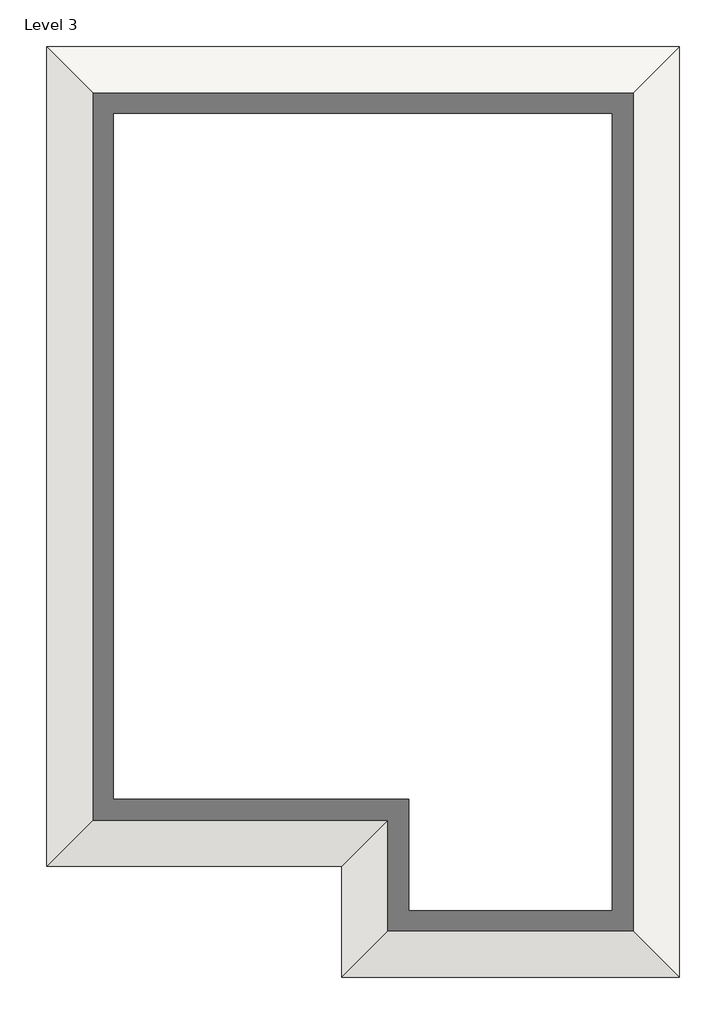
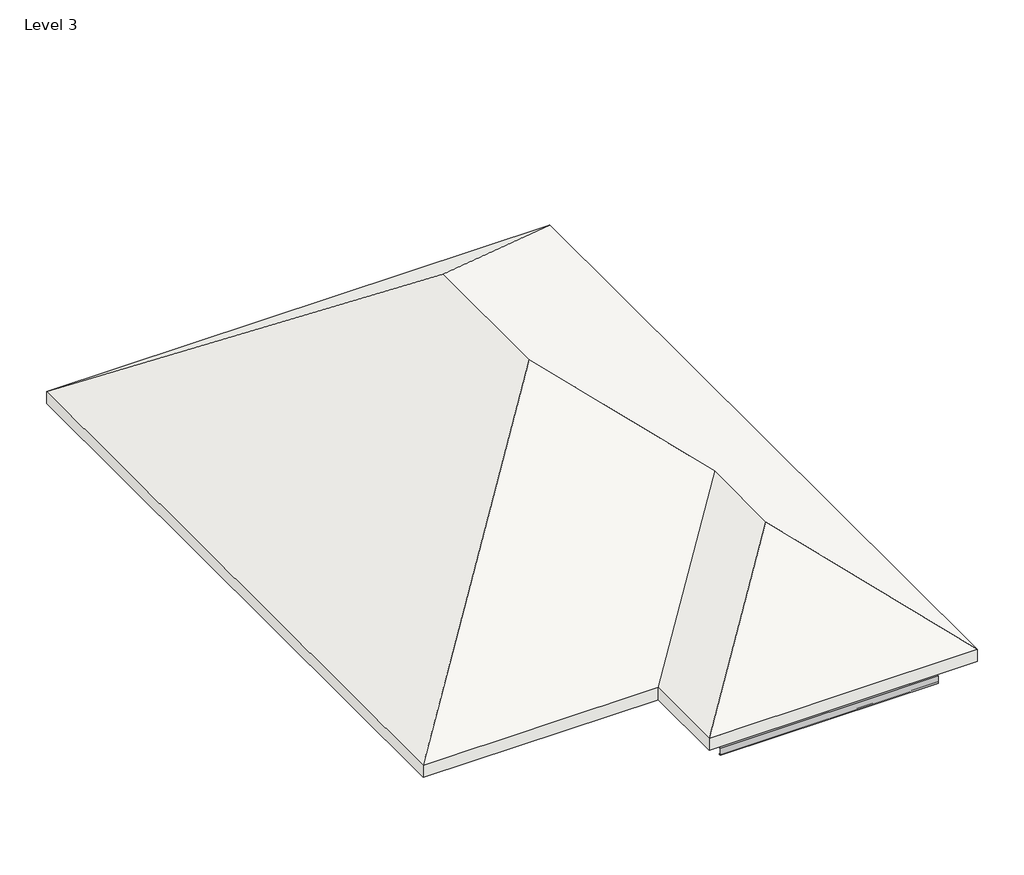
# One storey: 2 proxies, 1 roof.
"""IFC4 building model written with IfcOpenShell, lengths in millimetres."""

from ifc_helpers import new_model, si_unit, point, frame, frame_2d, origin, place, context, project, spatial, polyline, circle_curve, trimmed, segment, composite_curve, outline, extrude, faceted_brep, element, save

model = new_model("IFC4")

# Units and contexts
model_context = context("Model", 3, world=origin())
ifc_project = project(units=[si_unit("LENGTHUNIT", "METRE", prefix="MILLI")], contexts=[model_context])

# Site, building, storey
site = spatial("IfcSite", under=ifc_project)
building = spatial("IfcBuilding", under=site)
storey = spatial("IfcBuildingStorey", under=building, Name="Level 3", Elevation=6096.0)

# Proxies
placement = place(None, origin())
element("IfcBuildingElementProxy", 1, Name="Reveal", ObjectType="Reveal", at=placement, inside=storey, context=model_context, shape_type="SweptSolid", body=[
    extrude(outline(composite_curve([segment(polyline([(-10015.9757973, 5448.3), (-9952.7297973, 5448.3), (-9952.7297973, 5446.9203242)]), True, "CONTINUOUS"), segment(trimmed(circle_curve(frame_2d((-9957.9748973, 5446.9203242)), 5.2451), [point((-9952.7297973, 5446.9203242))], [point((-9957.1126065, 5441.7465897))], False, "CARTESIAN"), True, "CONTINUOUS"), segment(polyline([(-9957.1126065, 5441.7465897), (-9980.7332973, 5437.8098), (-9999.9711789, 5434.60348)]), True, "CONTINUOUS"), segment(trimmed(circle_curve(frame_2d((-9998.2465973, 5424.256011)), 10.4902), [point((-9999.9711789, 5434.60348))], [point((-10008.7367973, 5424.256011))], True, "CARTESIAN"), True, "CONTINUOUS"), segment(polyline([(-10008.7367973, 5424.256011), (-10008.7367973, 5243.743989)]), True, "CONTINUOUS"), segment(trimmed(circle_curve(frame_2d((-9998.2465973, 5243.743989)), 10.4902), [point((-10008.7367973, 5243.743989))], [point((-9999.9711789, 5233.39652))], True, "CARTESIAN"), True, "CONTINUOUS"), segment(polyline([(-9999.9711789, 5233.39652), (-9980.7332973, 5230.1902), (-9957.1126065, 5226.2534103)]), True, "CONTINUOUS"), segment(trimmed(circle_curve(frame_2d((-9957.9748973, 5221.0796758)), 5.2451), [point((-9957.1126065, 5226.2534103))], [point((-9952.7297973, 5221.0796758))], False, "CARTESIAN"), True, "CONTINUOUS"), segment(polyline([(-9952.7297973, 5221.0796758), (-9952.7297973, 5219.7), (-10015.9757973, 5219.7), (-10015.9757973, 5448.3)]), True, "CONTINUOUS")], self_intersect=False)), frame((-43748.9380314, 0.0, 0.0), z_axis=(1.0, 0.0, 0.0), x_axis=(0.0, 1.0, 0.0)), (0.0, 0.0, 1.0), 6502.4),
])
element("IfcBuildingElementProxy", 2, Name="Reveal", ObjectType="Reveal", at=placement, inside=storey, context=model_context, shape_type="SweptSolid", body=[
    extrude(outline(composite_curve([segment(polyline([(-10015.9757973, 6057.9), (-9952.7297973, 6057.9), (-9952.7297973, 6056.5203242)]), True, "CONTINUOUS"), segment(trimmed(circle_curve(frame_2d((-9957.9748973, 6056.5203242)), 5.2451), [point((-9952.7297973, 6056.5203242))], [point((-9957.1126065, 6051.3465897))], False, "CARTESIAN"), True, "CONTINUOUS"), segment(polyline([(-9957.1126065, 6051.3465897), (-9980.7332973, 6047.4098), (-9999.9711789, 6044.20348)]), True, "CONTINUOUS"), segment(trimmed(circle_curve(frame_2d((-9998.2465973, 6033.856011)), 10.4902), [point((-9999.9711789, 6044.20348))], [point((-10008.7367973, 6033.856011))], True, "CARTESIAN"), True, "CONTINUOUS"), segment(polyline([(-10008.7367973, 6033.856011), (-10008.7367973, 5853.343989)]), True, "CONTINUOUS"), segment(trimmed(circle_curve(frame_2d((-9998.2465973, 5853.343989)), 10.4902), [point((-10008.7367973, 5853.343989))], [point((-9999.9711789, 5842.99652))], True, "CARTESIAN"), True, "CONTINUOUS"), segment(polyline([(-9999.9711789, 5842.99652), (-9980.7332973, 5839.7902), (-9957.1126065, 5835.8534103)]), True, "CONTINUOUS"), segment(trimmed(circle_curve(frame_2d((-9957.9748973, 5830.6796758)), 5.2451), [point((-9957.1126065, 5835.8534103))], [point((-9952.7297973, 5830.6796758))], False, "CARTESIAN"), True, "CONTINUOUS"), segment(polyline([(-9952.7297973, 5830.6796758), (-9952.7297973, 5829.3), (-10015.9757973, 5829.3), (-10015.9757973, 6057.9)]), True, "CONTINUOUS")], self_intersect=False)), frame((-43748.9380314, 0.0, 0.0), z_axis=(1.0, 0.0, 0.0), x_axis=(0.0, 1.0, 0.0)), (0.0, 0.0, 1.0), 6502.4),
])

# Roof
element("IfcRoof", 3, ObjectType="roofing 1'", at=placement, inside=storey, context=model_context, shape_type="Brep", body=[
    faceted_brep([(-51521.3380314, -8121.4913973, 6096.0), (-51521.3380314, 11329.4990751, 6096.0), (-44015.6380314, 3823.7990751, 11725.275), (-44015.6380314, -615.7913973, 11725.275), (-40510.4380314, -4120.9913973, 9096.375), (-44510.9380314, -8121.4913973, 6096.0), (-44510.9380314, -10763.0913973, 6096.0), (-40510.4380314, -6762.5913973, 9096.375), (-36509.9380314, -10763.0913973, 6096.0), (-36509.9380314, 11329.4990751, 6096.0), (-51521.3380314, -8121.4913973, 6477.0), (-44015.6380314, -615.7913973, 12106.275), (-44015.6380314, 3823.7990751, 12106.275), (-51521.3380314, 11329.4990751, 6477.0), (-44510.9380314, -8121.4913973, 6477.0), (-40510.4380314, -4120.9913973, 9477.375), (-44510.9380314, -10763.0913973, 6477.0), (-40510.4380314, -6762.5913973, 9477.375), (-36509.9380314, -10763.0913973, 6477.0), (-36509.9380314, 11329.4990751, 6477.0)], [[[0, 1, 2, 3]], [[0, 3, 4, 5]], [[6, 5, 4, 7]], [[6, 7, 8]], [[9, 2, 1]], [[8, 7, 4, 3, 2, 9]], [[10, 11, 12, 13]], [[10, 14, 15, 11]], [[14, 16, 17, 15]], [[16, 18, 17]], [[19, 13, 12]], [[18, 19, 12, 11, 15, 17]], [[5, 14, 10, 0]], [[6, 16, 14, 5]], [[8, 18, 16, 6]], [[9, 19, 18, 8]], [[1, 13, 19, 9]], [[0, 10, 13, 1]]]),
])

save(model, "model.ifc")

# Revit data of these elements
# Type "roofing 1'"
#   Assembly Code = "B1020"
#   Layers, outside or top first: 1' - 0" "roofing" (function 1)
# Element 3 (IfcRoof, "roofing 1'")
#   built-in parameter 1001705 = 39.7187 (stored number, unit not read)
#   built-in parameter 1001710 = 33615
#   Phase Created = New Construction
#   Materials on its faces: "roofing"
# Materials
#   "roofing": class "Generic", colour RGB 120 120 120, transparency 0, Cost = 0
